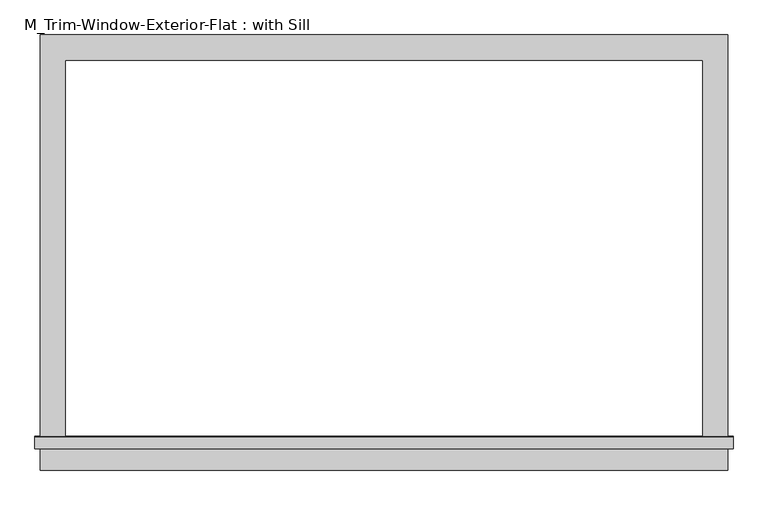
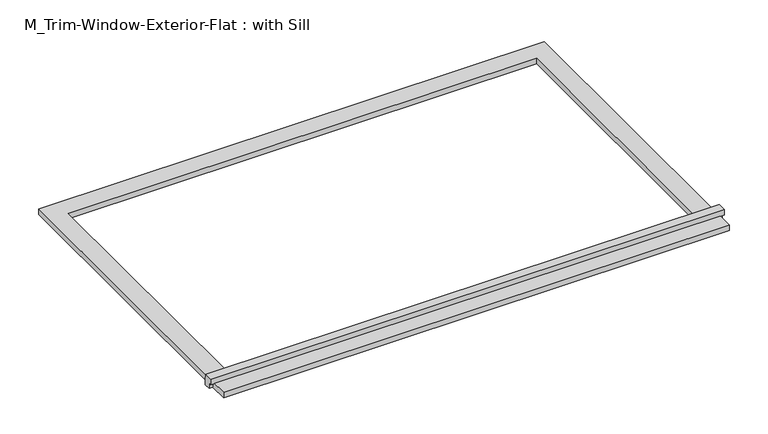
"""IFC4 building model written with IfcOpenShell, lengths in millimetres: proxy geometry, M_Trim-Window-Exterior-Flat : with Sill."""

from ifc_helpers import new_model, si_unit, frame, origin, origin_with_axes, place, context, project, spatial, polyline, outline, extrude, source, transform, mapped, element, save


def m_trim_window_exterior_flat_with_sill_30a8f3cc(model_context):
    return source(origin(), model_context, "Body", "SweptSolid", [
        extrude(outline(polyline([(822.0, -920.4323709), (822.0, -980.4323709), (-822.0, -980.4323709), (-822.0, -920.4323709), (822.0, -920.4323709)])), origin_with_axes(), (0.0, 0.0, 1.0), 19.05),
        extrude(outline(polyline([(-930.0, 38.1), (-902.4580645, 38.1), (-900.0, 19.05), (-900.0, 0.0), (-920.4323709, 0.0), (-920.4323709, 19.05), (-930.0, 19.05), (-930.0, 38.1)])), frame((-834.7, 0.0, 0.0), z_axis=(1.0, 0.0, 0.0), x_axis=(0.0, 1.0, 0.0)), (0.0, 0.0, 1.0), 1669.4),
        extrude(outline(polyline([(-822.0, 60.0), (822.0, 60.0), (822.0, -900.0), (762.0, -900.0), (762.0, 0.0), (-762.0, 0.0), (-762.0, -900.0), (-822.0, -900.0), (-822.0, 60.0)])), origin_with_axes(), (0.0, 0.0, 1.0), 19.05),
    ])


if __name__ == "__main__":
    model = new_model("IFC4")
    model_context = context("Model", 3, world=origin())
    ifc_project = project(units=[si_unit("LENGTHUNIT", "METRE", prefix="MILLI")], contexts=[model_context])
    site = spatial("IfcSite", under=ifc_project)
    building = spatial("IfcBuilding", under=site)
    placement = place(None, origin())
    m_trim_window_exterior_flat_with_sill_shape = m_trim_window_exterior_flat_with_sill_30a8f3cc(model_context)
    element("IfcBuildingElementProxy", 1, Name="M_Trim-Window-Exterior-Flat : with Sill", ObjectType="M_Trim-Window-Exterior-Flat : with Sill", at=placement, inside=building, context=model_context, shape_type="MappedRepresentation", body=[
        mapped(m_trim_window_exterior_flat_with_sill_shape, transform((0.0, 0.0, 0.0), x_axis=(1.0, 0.0, 0.0), y_axis=(0.0, 1.0, 0.0), z_axis=(0.0, 0.0, 1.0))),
    ])
    save(model, "model.ifc")

# Revit data of these elements
# Type "M_Trim-Window-Exterior-Flat : with Sill"
#   Trim Width = 0' - 2.3622"
#   Trim Thickness_Picture Frame = 0' - 1.1811"
#   Trim Thickness_with Sill = 0' - 0 3/4"
#   Sill Thickness = 0' - 1.1811"
#   Opening Width [instance default] = 1' - 11.62205"
#   Opening Height [instance default] = 2' - 11.43307"
#   Default Elevation = 3' - 11.24409"
#   Sill = yes
#   Picture Frame = no
#   Trim Material [instance default] = none
# Element 1 (IfcBuildingElementProxy, "M_Trim-Window-Exterior-Flat : with Sill")
#   Opening Width = 5' - 0"
#   Trim Material = Clad - White
#   Materials on its faces: "Clad - White"
# Materials
#   "Clad - White": class "Wood", colour RGB 242 242 238, transparency 0, Cost = 0
